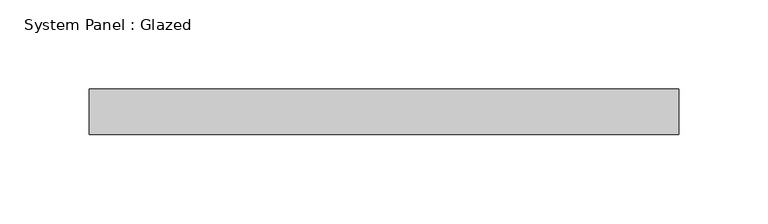
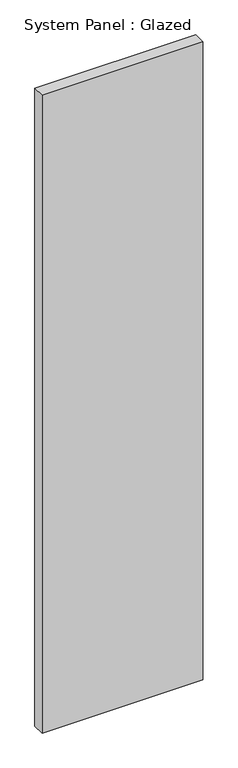
"""IFC4 building model written with IfcOpenShell, lengths in millimetres: plate geometry, System Panel : Glazed."""

from ifc_helpers import new_model, si_unit, origin, origin_with_axes, place, context, project, spatial, polyline, outline, extrude, source, transform, mapped, element, save


def system_panel_glazed_53ed24d2(model_context):
    return source(origin(), model_context, "Body", "SweptSolid", [
        extrude(outline(polyline([(165.1, 19.05), (-165.1, 19.05), (-165.1, 44.45), (165.1, 44.45), (165.1, 19.05)])), origin_with_axes(), (0.0, 0.0, 1.0), 1385.8617517),
    ])


if __name__ == "__main__":
    model = new_model("IFC4")
    model_context = context("Model", 3, world=origin())
    ifc_project = project(units=[si_unit("LENGTHUNIT", "METRE", prefix="MILLI")], contexts=[model_context])
    site = spatial("IfcSite", under=ifc_project)
    building = spatial("IfcBuilding", under=site)
    placement = place(None, origin())
    system_panel_glazed_shape = system_panel_glazed_53ed24d2(model_context)
    element("IfcPlate", 1, ObjectType="System Panel : Glazed", at=placement, inside=building, context=model_context, shape_type="MappedRepresentation", body=[
        mapped(system_panel_glazed_shape, transform((0.0, 0.0, 0.0), x_axis=(1.0, 0.0, 0.0), y_axis=(0.0, 1.0, 0.0), z_axis=(0.0, 0.0, 1.0))),
    ])
    save(model, "model.ifc")

# Revit data of these elements
# Type "System Panel : Glazed"
#   Construction Type Id = "GSP4R"
#   Analytic Construction = "1/8 in Pilkington single glazing"
#   Visual Light Transmittance = 0.9
#   Solar Heat Gain Coefficient = 0.86
#   Heat Transfer Coefficient (U) = 1.18115 BTU/(h·ft²·°F)
#   Define Thermal Properties by = 1
# Element 1 (IfcPlate, "System Panel : Glazed")
#   Materials on its faces: "Glass"
# Materials
#   "Glass": class "Glass", colour RGB 0 128 192, transparency 0.75, Description = "Soda Lime Glass", Cost = 0
